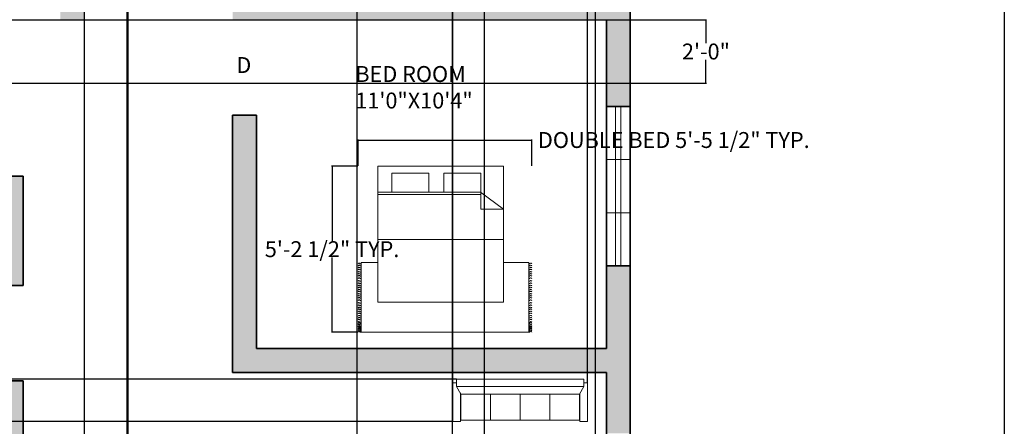
# Model space of a CAD drawing. Units: inches. Extents: x 2552 to 3196, y 4736 to 5443.
# Tile 4 of 8: x 2824 to 3196, y 4983 to 5136. Entities that reach past the tile are written whole.
import ezdxf

# ---------------------------------------------------------------- set-up
doc = ezdxf.new("R2010")
doc.units = ezdxf.units.IN
doc.header["$MEASUREMENT"] = 0
for name, color, linetype, lineweight in [('A-ANNO-DIMS', 2, 'Continuous', 18), ('A-ANNO-TTLB', 7, 'Continuous', 25), ('A-AREA-IDEN', 7, 'Continuous', 18), ('A-DOOR-IDEN', 7, 'Continuous', 18), ('A-FURN', 8, 'Continuous', 18), ('A-GLAZ', 4, 'Continuous', 18), ('A-WALL', 7, 'Continuous', 35)]:
    doc.layers.add(name, color=color, linetype=linetype, lineweight=lineweight)
doc.layers.add('A-WALL-PATT', color=30, linetype='Continuous', lineweight=13, true_color=0xf8991e)
doc.styles.get("Standard").update_dxf_attribs({"font": 'arial.ttf'})
doc.dimstyles.get("Standard").update_dxf_attribs({"dimtxt": 6, "dimasz": 0.18, "dimexe": 0.18, "dimexo": 0.0625, "dimgap": 0.09, "dimtad": 0, "dimtih": 1, "dimtoh": 1, "dimdec": 1, "dimzin": 0, "dimdsep": 46, "dimlunit": 3, "dimtxsty": 'Standard', "dimcen": 0.09, "dimadec": 0, "dimazin": 0, "dimtfac": 1, "dimtdec": 1, "dimtofl": 0, "dimtmove": 0, "dimatfit": 3, "dimfxl": 1, "dimtolj": 1, "dimtzin": 0, "dimarcsym": 0})

# ---------------------------------------------------------------- blocks, each defined once
blk = doc.blocks.new('WIN-60IN-THREE-LIGHT')
for p, q in [((60, 9), (0, 9)), ((20, 9), (20, 0)), ((40, 0), (40, 9)), ((60, 5.5), (0, 5.5)), ((0, 3.5), (60, 3.5)), ((0, 0), (60, 0))]:
    blk.add_line(p, q)
blk = doc.blocks.new('BED-DOUBLE')
for p, q in [((46.16, 52.82), (7.4, 52.82)), ((46.22, 52), (7.4, 52)), ((46.16, 52.82), (54.77, 46.47)), ((46.22, 52.82), (46.22, 46.47)), ((46.22, 46.47), (54.77, 46.47)), ((54.83, 34.96), (7.4, 34.96)), ((1.13, 0), (1.13, 26.37)), ((1.13, 26.37), (7.43, 26.37)), ((54.83, 26.37), (64.37, 26.37)), ((64.37, 26.37), (64.37, 0)), ((64.37, 0), (1.13, 0))]:
    blk.add_line(p, q)
for points in [[(54.83, 62.68), (54.83, 11.36), (7.4, 11.36), (7.4, 62.68)], [(26.65, 59.98), (26.65, 52.82), (12.75, 52.82), (12.75, 59.98)], [(46.22, 59.98), (46.22, 52.82), (32.32, 52.82), (32.32, 59.98)]]:
    blk.add_lwpolyline(points, close=True)
for points, knots in [([(0, 25.83), (0.1, 25.96), (0.29, 26.2), (0.63, 25.96), (0.91, 25.78), (1.06, 25.89), (1.13, 25.94)], [0, 0, 0, 0, 0.400747, 0.791423, 1.067667, 1.29709, 1.29709, 1.29709, 1.29709]), ([(65.48, 25.83), (65.39, 25.96), (65.19, 26.2), (64.85, 25.96), (64.57, 25.78), (64.42, 25.89), (64.36, 25.94)], [0, 0, 0, 0, 0.400747, 0.791423, 1.067667, 1.29709, 1.29709, 1.29709, 1.29709]), ([(0, 25.06), (0.1, 25.18), (0.29, 25.42), (0.63, 25.18), (0.91, 25), (1.06, 25.11), (1.13, 25.16)], [0, 0, 0, 0, 0.400747, 0.791423, 1.067667, 1.29709, 1.29709, 1.29709, 1.29709]), ([(0, 24.24), (0.1, 24.36), (0.29, 24.6), (0.63, 24.36), (0.91, 24.19), (1.06, 24.29), (1.13, 24.34)], [0, 0, 0, 0, 0.400747, 0.791423, 1.067667, 1.29709, 1.29709, 1.29709, 1.29709]), ([(0, 23.51), (0.1, 23.63), (0.29, 23.87), (0.63, 23.63), (0.91, 23.46), (1.06, 23.57), (1.13, 23.62)], [0, 0, 0, 0, 0.400747, 0.791423, 1.067667, 1.29709, 1.29709, 1.29709, 1.29709]), ([(0, 22.63), (0.1, 22.75), (0.29, 22.99), (0.63, 22.75), (0.91, 22.58), (1.06, 22.68), (1.13, 22.73)], [0, 0, 0, 0, 0.400747, 0.791423, 1.067667, 1.29709, 1.29709, 1.29709, 1.29709]), ([(65.48, 25.06), (65.39, 25.18), (65.19, 25.42), (64.85, 25.18), (64.57, 25), (64.42, 25.11), (64.36, 25.16)], [0, 0, 0, 0, 0.400747, 0.791423, 1.067667, 1.29709, 1.29709, 1.29709, 1.29709]), ([(65.48, 24.24), (65.39, 24.36), (65.19, 24.6), (64.85, 24.36), (64.57, 24.19), (64.42, 24.29), (64.36, 24.34)], [0, 0, 0, 0, 0.400747, 0.791423, 1.067667, 1.29709, 1.29709, 1.29709, 1.29709]), ([(65.48, 23.51), (65.39, 23.63), (65.19, 23.87), (64.85, 23.63), (64.57, 23.46), (64.42, 23.57), (64.36, 23.62)], [0, 0, 0, 0, 0.400747, 0.791423, 1.067667, 1.29709, 1.29709, 1.29709, 1.29709]), ([(65.48, 22.63), (65.39, 22.75), (65.19, 22.99), (64.85, 22.75), (64.57, 22.58), (64.42, 22.68), (64.36, 22.73)], [0, 0, 0, 0, 0.400747, 0.791423, 1.067667, 1.29709, 1.29709, 1.29709, 1.29709]), ([(0, 21.88), (0.1, 22), (0.29, 22.24), (0.63, 22), (0.91, 21.83), (1.06, 21.93), (1.13, 21.98)], [0, 0, 0, 0, 0.400747, 0.791423, 1.067667, 1.29709, 1.29709, 1.29709, 1.29709]), ([(0, 21.15), (0.1, 21.27), (0.29, 21.51), (0.63, 21.27), (0.91, 21.1), (1.06, 21.2), (1.13, 21.25)], [0, 0, 0, 0, 0.400747, 0.791423, 1.067667, 1.29709, 1.29709, 1.29709, 1.29709]), ([(0, 20.27), (0.1, 20.39), (0.29, 20.63), (0.63, 20.39), (0.91, 20.22), (1.06, 20.32), (1.13, 20.37)], [0, 0, 0, 0, 0.400747, 0.791423, 1.067667, 1.29709, 1.29709, 1.29709, 1.29709]), ([(0, 19.23), (0.1, 19.35), (0.29, 19.59), (0.63, 19.35), (0.91, 19.18), (1.06, 19.29), (1.13, 19.33)], [0, 0, 0, 0, 0.400747, 0.791423, 1.067667, 1.29709, 1.29709, 1.29709, 1.29709]), ([(0, 18.35), (0.1, 18.47), (0.29, 18.71), (0.63, 18.47), (0.91, 18.3), (1.06, 18.4), (1.13, 18.45)], [0, 0, 0, 0, 0.400747, 0.791423, 1.067667, 1.29709, 1.29709, 1.29709, 1.29709]), ([(65.48, 21.88), (65.39, 22), (65.19, 22.24), (64.85, 22), (64.57, 21.83), (64.42, 21.93), (64.36, 21.98)], [0, 0, 0, 0, 0.400747, 0.791423, 1.067667, 1.29709, 1.29709, 1.29709, 1.29709]), ([(65.48, 21.15), (65.39, 21.27), (65.19, 21.51), (64.85, 21.27), (64.57, 21.1), (64.42, 21.2), (64.36, 21.25)], [0, 0, 0, 0, 0.400747, 0.791423, 1.067667, 1.29709, 1.29709, 1.29709, 1.29709]), ([(65.48, 20.27), (65.39, 20.39), (65.19, 20.63), (64.85, 20.39), (64.57, 20.22), (64.42, 20.32), (64.36, 20.37)], [0, 0, 0, 0, 0.400747, 0.791423, 1.067667, 1.29709, 1.29709, 1.29709, 1.29709]), ([(65.48, 19.23), (65.39, 19.35), (65.19, 19.59), (64.85, 19.35), (64.57, 19.18), (64.42, 19.29), (64.36, 19.33)], [0, 0, 0, 0, 0.400747, 0.791423, 1.067667, 1.29709, 1.29709, 1.29709, 1.29709]), ([(65.48, 18.35), (65.39, 18.47), (65.19, 18.71), (64.85, 18.47), (64.57, 18.3), (64.42, 18.4), (64.36, 18.45)], [0, 0, 0, 0, 0.400747, 0.791423, 1.067667, 1.29709, 1.29709, 1.29709, 1.29709]), ([(0, 17.53), (0.1, 17.65), (0.29, 17.89), (0.63, 17.65), (0.91, 17.48), (1.06, 17.59), (1.13, 17.64)], [0, 0, 0, 0, 0.400747, 0.791423, 1.067667, 1.29709, 1.29709, 1.29709, 1.29709]), ([(0, 16.76), (0.1, 16.88), (0.29, 17.12), (0.63, 16.88), (0.91, 16.7), (1.06, 16.81), (1.13, 16.86)], [0, 0, 0, 0, 0.400747, 0.791423, 1.067667, 1.29709, 1.29709, 1.29709, 1.29709]), ([(0, 15.94), (0.1, 16.06), (0.29, 16.3), (0.63, 16.06), (0.91, 15.89), (1.06, 15.99), (1.13, 16.04)], [0, 0, 0, 0, 0.400747, 0.791423, 1.067667, 1.29709, 1.29709, 1.29709, 1.29709]), ([(0, 15.21), (0.1, 15.33), (0.29, 15.57), (0.63, 15.33), (0.91, 15.16), (1.06, 15.27), (1.13, 15.31)], [0, 0, 0, 0, 0.400747, 0.791423, 1.067667, 1.29709, 1.29709, 1.29709, 1.29709]), ([(65.48, 17.53), (65.39, 17.65), (65.19, 17.89), (64.85, 17.65), (64.57, 17.48), (64.42, 17.59), (64.36, 17.64)], [0, 0, 0, 0, 0.400747, 0.791423, 1.067667, 1.29709, 1.29709, 1.29709, 1.29709]), ([(65.48, 16.76), (65.39, 16.88), (65.19, 17.12), (64.85, 16.88), (64.57, 16.7), (64.42, 16.81), (64.36, 16.86)], [0, 0, 0, 0, 0.400747, 0.791423, 1.067667, 1.29709, 1.29709, 1.29709, 1.29709]), ([(65.48, 15.94), (65.39, 16.06), (65.19, 16.3), (64.85, 16.06), (64.57, 15.89), (64.42, 15.99), (64.36, 16.04)], [0, 0, 0, 0, 0.400747, 0.791423, 1.067667, 1.29709, 1.29709, 1.29709, 1.29709]), ([(65.48, 15.21), (65.39, 15.33), (65.19, 15.57), (64.85, 15.33), (64.57, 15.16), (64.42, 15.27), (64.36, 15.31)], [0, 0, 0, 0, 0.400747, 0.791423, 1.067667, 1.29709, 1.29709, 1.29709, 1.29709]), ([(0, 14.33), (0.1, 14.45), (0.29, 14.69), (0.63, 14.45), (0.91, 14.28), (1.06, 14.38), (1.13, 14.43)], [0, 0, 0, 0, 0.400747, 0.791423, 1.067667, 1.29709, 1.29709, 1.29709, 1.29709]), ([(0, 13.58), (0.1, 13.7), (0.29, 13.94), (0.63, 13.7), (0.91, 13.53), (1.06, 13.63), (1.13, 13.68)], [0, 0, 0, 0, 0.400747, 0.791423, 1.067667, 1.29709, 1.29709, 1.29709, 1.29709]), ([(0, 12.85), (0.1, 12.97), (0.29, 13.21), (0.63, 12.97), (0.91, 12.8), (1.06, 12.9), (1.13, 12.95)], [0, 0, 0, 0, 0.400747, 0.791423, 1.067667, 1.29709, 1.29709, 1.29709, 1.29709]), ([(0, 11.97), (0.1, 12.09), (0.29, 12.33), (0.63, 12.09), (0.91, 11.92), (1.06, 12.02), (1.13, 12.07)], [0, 0, 0, 0, 0.400747, 0.791423, 1.067667, 1.29709, 1.29709, 1.29709, 1.29709]), ([(0, 10.93), (0.1, 11.05), (0.29, 11.29), (0.63, 11.05), (0.91, 10.88), (1.06, 10.99), (1.13, 11.03)], [0, 0, 0, 0, 0.400747, 0.791423, 1.067667, 1.29709, 1.29709, 1.29709, 1.29709]), ([(65.48, 14.33), (65.39, 14.45), (65.19, 14.69), (64.85, 14.45), (64.57, 14.28), (64.42, 14.38), (64.36, 14.43)], [0, 0, 0, 0, 0.400747, 0.791423, 1.067667, 1.29709, 1.29709, 1.29709, 1.29709]), ([(65.48, 13.58), (65.39, 13.7), (65.19, 13.94), (64.85, 13.7), (64.57, 13.53), (64.42, 13.63), (64.36, 13.68)], [0, 0, 0, 0, 0.400747, 0.791423, 1.067667, 1.29709, 1.29709, 1.29709, 1.29709]), ([(65.48, 12.85), (65.39, 12.97), (65.19, 13.21), (64.85, 12.97), (64.57, 12.8), (64.42, 12.9), (64.36, 12.95)], [0, 0, 0, 0, 0.400747, 0.791423, 1.067667, 1.29709, 1.29709, 1.29709, 1.29709]), ([(65.48, 11.97), (65.39, 12.09), (65.19, 12.33), (64.85, 12.09), (64.57, 11.92), (64.42, 12.02), (64.36, 12.07)], [0, 0, 0, 0, 0.400747, 0.791423, 1.067667, 1.29709, 1.29709, 1.29709, 1.29709]), ([(65.48, 10.93), (65.39, 11.05), (65.19, 11.29), (64.85, 11.05), (64.57, 10.88), (64.42, 10.99), (64.36, 11.03)], [0, 0, 0, 0, 0.400747, 0.791423, 1.067667, 1.29709, 1.29709, 1.29709, 1.29709]), ([(0, 10.05), (0.1, 10.17), (0.29, 10.41), (0.63, 10.17), (0.91, 10), (1.06, 10.1), (1.13, 10.15)], [0, 0, 0, 0, 0.400747, 0.791423, 1.067667, 1.29709, 1.29709, 1.29709, 1.29709]), ([(0, 9.23), (0.1, 9.35), (0.29, 9.59), (0.63, 9.35), (0.91, 9.18), (1.06, 9.29), (1.13, 9.33)], [0, 0, 0, 0, 0.400747, 0.791423, 1.067667, 1.29709, 1.29709, 1.29709, 1.29709]), ([(0, 8.54), (0.1, 8.66), (0.29, 8.9), (0.63, 8.66), (0.91, 8.49), (1.06, 8.6), (1.13, 8.65)], [0, 0, 0, 0, 0.400747, 0.791423, 1.067667, 1.29709, 1.29709, 1.29709, 1.29709]), ([(0, 7.73), (0.1, 7.85), (0.29, 8.09), (0.63, 7.85), (0.91, 7.67), (1.06, 7.78), (1.13, 7.83)], [0, 0, 0, 0, 0.400747, 0.791423, 1.067667, 1.29709, 1.29709, 1.29709, 1.29709]), ([(65.48, 10.05), (65.39, 10.17), (65.19, 10.41), (64.85, 10.17), (64.57, 10), (64.42, 10.1), (64.36, 10.15)], [0, 0, 0, 0, 0.400747, 0.791423, 1.067667, 1.29709, 1.29709, 1.29709, 1.29709]), ([(65.48, 9.23), (65.39, 9.35), (65.19, 9.59), (64.85, 9.35), (64.57, 9.18), (64.42, 9.29), (64.36, 9.33)], [0, 0, 0, 0, 0.400747, 0.791423, 1.067667, 1.29709, 1.29709, 1.29709, 1.29709]), ([(65.48, 8.54), (65.39, 8.66), (65.19, 8.9), (64.85, 8.66), (64.57, 8.49), (64.42, 8.6), (64.36, 8.65)], [0, 0, 0, 0, 0.400747, 0.791423, 1.067667, 1.29709, 1.29709, 1.29709, 1.29709]), ([(65.48, 7.73), (65.39, 7.85), (65.19, 8.09), (64.85, 7.85), (64.57, 7.67), (64.42, 7.78), (64.36, 7.83)], [0, 0, 0, 0, 0.400747, 0.791423, 1.067667, 1.29709, 1.29709, 1.29709, 1.29709]), ([(0, 7), (0.1, 7.12), (0.29, 7.36), (0.63, 7.12), (0.91, 6.95), (1.06, 7.05), (1.13, 7.1)], [0, 0, 0, 0, 0.400747, 0.791423, 1.067667, 1.29709, 1.29709, 1.29709, 1.29709]), ([(0, 6.12), (0.1, 6.24), (0.29, 6.48), (0.63, 6.24), (0.91, 6.06), (1.06, 6.17), (1.13, 6.22)], [0, 0, 0, 0, 0.400747, 0.791423, 1.067667, 1.29709, 1.29709, 1.29709, 1.29709]), ([(0, 5.36), (0.1, 5.49), (0.29, 5.72), (0.63, 5.49), (0.91, 5.31), (1.06, 5.42), (1.13, 5.47)], [0, 0, 0, 0, 0.400747, 0.791423, 1.067667, 1.29709, 1.29709, 1.29709, 1.29709]), ([(0, 4.64), (0.1, 4.76), (0.29, 5), (0.63, 4.76), (0.91, 4.58), (1.06, 4.69), (1.13, 4.74)], [0, 0, 0, 0, 0.400747, 0.791423, 1.067667, 1.29709, 1.29709, 1.29709, 1.29709]), ([(0, 3.75), (0.1, 3.87), (0.29, 4.11), (0.63, 3.87), (0.91, 3.7), (1.06, 3.81), (1.13, 3.86)], [0, 0, 0, 0, 0.400747, 0.791423, 1.067667, 1.29709, 1.29709, 1.29709, 1.29709]), ([(65.48, 7), (65.39, 7.12), (65.19, 7.36), (64.85, 7.12), (64.57, 6.95), (64.42, 7.05), (64.36, 7.1)], [0, 0, 0, 0, 0.400747, 0.791423, 1.067667, 1.29709, 1.29709, 1.29709, 1.29709]), ([(65.48, 6.12), (65.39, 6.24), (65.19, 6.48), (64.85, 6.24), (64.57, 6.06), (64.42, 6.17), (64.36, 6.22)], [0, 0, 0, 0, 0.400747, 0.791423, 1.067667, 1.29709, 1.29709, 1.29709, 1.29709]), ([(65.48, 5.36), (65.39, 5.49), (65.19, 5.72), (64.85, 5.49), (64.57, 5.31), (64.42, 5.42), (64.36, 5.47)], [0, 0, 0, 0, 0.400747, 0.791423, 1.067667, 1.29709, 1.29709, 1.29709, 1.29709]), ([(65.48, 4.64), (65.39, 4.76), (65.19, 5), (64.85, 4.76), (64.58, 4.59), (64.43, 4.69), (64.37, 4.73)], [0, 0, 0, 0, 0.400747, 0.791423, 1.067667, 1.283686, 1.283686, 1.283686, 1.283686]), ([(65.48, 3.75), (65.39, 3.87), (65.19, 4.11), (64.85, 3.88), (64.58, 3.7), (64.43, 3.8), (64.37, 3.85)], [0, 0, 0, 0, 0.400747, 0.791423, 1.067667, 1.283686, 1.283686, 1.283686, 1.283686]), ([(0, 3.32), (0.1, 3.45), (0.29, 3.7), (0.63, 3.44), (0.91, 3.27), (1.06, 3.38), (1.13, 3.43)], [0, 0, 0, 0, 0.407265, 0.802015, 1.07826, 1.307683, 1.307683, 1.307683, 1.307683]), ([(0, 2.76), (0.1, 2.88), (0.29, 3.12), (0.63, 2.88), (0.91, 2.71), (1.06, 2.81), (1.13, 2.86)], [0, 0, 0, 0, 0.400747, 0.791423, 1.067667, 1.29709, 1.29709, 1.29709, 1.29709]), ([(0, 2.18), (0.1, 2.31), (0.29, 2.54), (0.63, 2.31), (0.91, 2.13), (1.06, 2.24), (1.13, 2.29)], [0, 0, 0, 0, 0.400747, 0.791423, 1.067667, 1.29709, 1.29709, 1.29709, 1.29709]), ([(0, 1.88), (0.1, 2), (0.29, 2.24), (0.63, 2), (0.91, 1.82), (1.06, 1.93), (1.13, 1.98)], [0, 0, 0, 0, 0.400747, 0.791423, 1.067667, 1.29709, 1.29709, 1.29709, 1.29709]), ([(0, 1.46), (0.1, 1.58), (0.29, 1.82), (0.63, 1.58), (0.91, 1.4), (1.06, 1.51), (1.13, 1.56)], [0, 0, 0, 0, 0.400747, 0.791423, 1.067667, 1.29709, 1.29709, 1.29709, 1.29709]), ([(0, 1.06), (0.1, 1.18), (0.29, 1.42), (0.63, 1.18), (0.91, 1.01), (1.06, 1.11), (1.13, 1.16)], [0, 0, 0, 0, 0.400747, 0.791423, 1.067667, 1.29709, 1.29709, 1.29709, 1.29709]), ([(0, 0.57), (0.1, 0.7), (0.29, 0.93), (0.63, 0.7), (0.91, 0.52), (1.06, 0.63), (1.13, 0.68)], [0, 0, 0, 0, 0.400747, 0.791423, 1.067667, 1.29709, 1.29709, 1.29709, 1.29709]), ([(0, 0.07), (0.1, 0.19), (0.29, 0.43), (0.63, 0.19), (0.91, 0.02), (1.06, 0.13), (1.13, 0.17)], [0, 0, 0, 0, 0.400747, 0.791423, 1.067667, 1.29709, 1.29709, 1.29709, 1.29709]), ([(65.48, 1.43), (65.39, 1.55), (65.19, 1.79), (64.85, 1.55), (64.57, 1.38), (64.42, 1.48), (64.36, 1.53)], [0, 0, 0, 0, 0.400747, 0.791423, 1.067667, 1.29709, 1.29709, 1.29709, 1.29709]), ([(65.48, 1.03), (65.39, 1.15), (65.19, 1.39), (64.85, 1.15), (64.57, 0.98), (64.42, 1.09), (64.36, 1.13)], [0, 0, 0, 0, 0.400747, 0.791423, 1.067667, 1.29709, 1.29709, 1.29709, 1.29709]), ([(65.48, 0.55), (65.39, 0.67), (65.19, 0.91), (64.85, 0.67), (64.57, 0.49), (64.42, 0.6), (64.36, 0.65)], [0, 0, 0, 0, 0.400747, 0.791423, 1.067667, 1.29709, 1.29709, 1.29709, 1.29709]), ([(65.48, 0.07), (65.39, 0.19), (65.19, 0.43), (64.85, 0.19), (64.57, 0.02), (64.42, 0.13), (64.36, 0.17)], [0, 0, 0, 0, 0.400747, 0.791423, 1.067667, 1.29709, 1.29709, 1.29709, 1.29709]), ([(65.48, 3.32), (65.39, 3.45), (65.19, 3.69), (64.85, 3.45), (64.58, 3.27), (64.43, 3.37), (64.37, 3.42)], [0, 0, 0, 0, 0.402903, 0.794912, 1.071156, 1.287177, 1.287177, 1.287177, 1.287177]), ([(65.48, 2.73), (65.39, 2.85), (65.19, 3.09), (64.85, 2.85), (64.58, 2.68), (64.43, 2.78), (64.37, 2.82)], [0, 0, 0, 0, 0.400747, 0.791423, 1.067667, 1.283686, 1.283686, 1.283686, 1.283686]), ([(65.48, 2.16), (65.39, 2.28), (65.19, 2.52), (64.85, 2.28), (64.58, 2.11), (64.43, 2.21), (64.37, 2.25)], [0, 0, 0, 0, 0.400747, 0.791423, 1.067667, 1.283686, 1.283686, 1.283686, 1.283686]), ([(65.48, 1.85), (65.39, 1.97), (65.19, 2.21), (64.85, 1.97), (64.58, 1.8), (64.43, 1.9), (64.37, 1.94)], [0, 0, 0, 0, 0.400747, 0.791423, 1.067667, 1.283686, 1.283686, 1.283686, 1.283686])]:
    blk.add_open_spline(points, degree=3, knots=knots)
blk = doc.blocks.new('*D13')
at = {"layer": 'A-ANNO-DIMS', "color": 0, "lineweight": -2, "transparency": 16777216}
for p, q in [((2952.04, 5081.18), (2952.04, 5091.12)), ((2952.22, 5090.94), (3017.34, 5090.94)), ((3017.52, 5081.18), (3017.52, 5091.12)), ((3017.52, 5090.94), (3017.7, 5090.94))]:
    blk.add_line(p, q, dxfattribs=at)
at = {"layer": 'A-ANNO-DIMS', "color": 0, "transparency": 16777216}
for points in [[(2952.22, 5090.97), (2952.22, 5090.91), (2952.04, 5090.94)], [(3017.34, 5090.97), (3017.34, 5090.91), (3017.52, 5090.94)]]:
    blk.add_solid(points, dxfattribs=at)
at = {"layer": 'Defpoints', "color": 0, "transparency": 16777216}
for p in [(3017.52, 5090.94), (2952.04, 5081.12), (3017.52, 5081.12)]:
    blk.add_point(p, dxfattribs=at)
at = {"layer": 'A-ANNO-DIMS', "color": 0, "transparency": 16777216, "insert": (3071.1, 5090.94), "char_height": 6, "attachment_point": 5}
blk.add_mtext('\\A1;DOUBLE BED 5\'-5 1/2" TYP.', dxfattribs=at)
blk = doc.blocks.new('*D14')
at = {"layer": 'A-ANNO-DIMS', "color": 0, "lineweight": -2, "transparency": 16777216}
for p, q in [((2951.97, 5081.12), (2942.03, 5081.12)), ((2942.21, 5080.94), (2942.21, 5052.97)), ((2942.21, 5018.62), (2942.21, 5046.59)), ((2951.97, 5018.44), (2942.03, 5018.44))]:
    blk.add_line(p, q, dxfattribs=at)
at = {"layer": 'A-ANNO-DIMS', "color": 0, "transparency": 16777216}
for points in [[(2942.18, 5080.94), (2942.24, 5080.94), (2942.21, 5081.12)], [(2942.18, 5018.62), (2942.24, 5018.62), (2942.21, 5018.44)]]:
    blk.add_solid(points, dxfattribs=at)
at = {"layer": 'Defpoints', "color": 0, "transparency": 16777216}
for p in [(2942.21, 5081.12), (2952.04, 5081.12), (2952.04, 5018.44)]:
    blk.add_point(p, dxfattribs=at)
at = {"layer": 'A-ANNO-DIMS', "color": 0, "transparency": 16777216, "insert": (2942.21, 5049.78), "char_height": 6, "attachment_point": 5}
blk.add_mtext('\\A1;5\'-2 1/2" TYP.', dxfattribs=at)
blk = doc.blocks.new('*D24')
at = {"layer": 'A-ANNO-DIMS', "color": 0, "lineweight": -2, "transparency": 16777216}
for p, q in [((2951.66, 4886.38), (2951.66, 5320.05)), ((2951.84, 5319.87), (2961.59, 5319.87)), ((2987.48, 5319.87), (2977.72, 5319.87)), ((2987.66, 4886.38), (2987.66, 5320.05))]:
    blk.add_line(p, q, dxfattribs=at)
at = {"layer": 'A-ANNO-DIMS', "color": 0, "transparency": 16777216}
for points in [[(2951.84, 5319.9), (2951.84, 5319.84), (2951.66, 5319.87)], [(2987.48, 5319.9), (2987.48, 5319.84), (2987.66, 5319.87)]]:
    blk.add_solid(points, dxfattribs=at)
at = {"layer": 'Defpoints', "color": 0, "transparency": 16777216}
for p in [(2987.66, 5319.87), (2951.66, 4886.32), (2987.66, 4886.32)]:
    blk.add_point(p, dxfattribs=at)
at = {"layer": 'A-ANNO-DIMS', "color": 0, "transparency": 16777216, "insert": (2969.66, 5319.87), "char_height": 6, "attachment_point": 5}
blk.add_mtext('\\A1;3\'-0"', dxfattribs=at)
blk = doc.blocks.new('*D26')
at = {"layer": 'A-ANNO-DIMS', "color": 0, "lineweight": -2, "transparency": 16777216}
for p, q in [((2803.72, 5136.32), (3083.39, 5136.32)), ((3083.21, 5136.14), (3083.21, 5127.47)), ((3083.21, 5112.5), (3083.21, 5121.16)), ((2773.72, 5112.32), (3083.39, 5112.32))]:
    blk.add_line(p, q, dxfattribs=at)
at = {"layer": 'A-ANNO-DIMS', "color": 0, "transparency": 16777216}
for points in [[(3083.18, 5136.14), (3083.24, 5136.14), (3083.21, 5136.32)], [(3083.18, 5112.5), (3083.24, 5112.5), (3083.21, 5112.32)]]:
    blk.add_solid(points, dxfattribs=at)
at = {"layer": 'Defpoints', "color": 0, "transparency": 16777216}
for p in [(2803.66, 5136.32), (2773.66, 5112.32), (3083.21, 5112.32)]:
    blk.add_point(p, dxfattribs=at)
at = {"layer": 'A-ANNO-DIMS', "color": 0, "transparency": 16777216, "insert": (3083.21, 5124.32), "char_height": 6, "attachment_point": 5}
blk.add_mtext('\\A1;2\'-0"', dxfattribs=at)
blk = doc.blocks.new('*D27')
at = {"layer": 'A-ANNO-DIMS', "color": 0, "lineweight": -2, "transparency": 16777216}
for p, q in [((2999.73, 4817.38), (2999.73, 5320.05)), ((2999.91, 5319.87), (3012.6, 5319.87)), ((3041.41, 5319.87), (3028.73, 5319.87)), ((3041.59, 4817.38), (3041.59, 5320.05))]:
    blk.add_line(p, q, dxfattribs=at)
at = {"layer": 'A-ANNO-DIMS', "color": 0, "transparency": 16777216}
for points in [[(2999.91, 5319.9), (2999.91, 5319.84), (2999.73, 5319.87)], [(3041.41, 5319.9), (3041.41, 5319.84), (3041.59, 5319.87)]]:
    blk.add_solid(points, dxfattribs=at)
at = {"layer": 'Defpoints', "color": 0, "transparency": 16777216}
for p in [(3041.59, 5319.87), (2999.73, 4817.32), (3041.59, 4817.32)]:
    blk.add_point(p, dxfattribs=at)
at = {"layer": 'A-ANNO-DIMS', "color": 0, "transparency": 16777216, "insert": (3020.66, 5319.87), "char_height": 6, "attachment_point": 5}
blk.add_mtext('\\A1;3\'-6"', dxfattribs=at)
blk = doc.blocks.new('*D31')
at = {"layer": 'A-ANNO-DIMS', "color": 0, "lineweight": -2, "transparency": 16777216}
for p, q in [((2848.66, 5282.26), (2848.66, 4759.59)), ((2865.22, 5282.26), (2865.22, 4759.59)), ((2848.84, 4759.77), (2865.04, 4759.77)), ((2865.22, 4759.77), (2865.4, 4759.77))]:
    blk.add_line(p, q, dxfattribs=at)
at = {"layer": 'A-ANNO-DIMS', "color": 0, "transparency": 16777216}
for points in [[(2848.84, 4759.8), (2848.84, 4759.74), (2848.66, 4759.77)], [(2865.04, 4759.8), (2865.04, 4759.74), (2865.22, 4759.77)]]:
    blk.add_solid(points, dxfattribs=at)
at = {"layer": 'Defpoints', "color": 0, "transparency": 16777216}
for p in [(2848.66, 5282.32), (2865.22, 5282.32), (2865.22, 4759.77)]:
    blk.add_point(p, dxfattribs=at)
at = {"layer": 'A-ANNO-DIMS', "color": 0, "transparency": 16777216, "insert": (2880.18, 4759.77), "char_height": 6, "attachment_point": 5}
blk.add_mtext('\\A1;1\'-4 1/2"', dxfattribs=at)
blk = doc.blocks.new('*D32')
at = {"layer": 'A-ANNO-DIMS', "color": 0, "lineweight": -2, "transparency": 16777216}
for p, q in [((2864.75, 5194.1), (2864.75, 4759.59)), ((2848.66, 5191.26), (2848.66, 4759.59)), ((2848.48, 4759.77), (2848.3, 4759.77)), ((2864.93, 4759.77), (2865.11, 4759.77))]:
    blk.add_line(p, q, dxfattribs=at)
at = {"layer": 'A-ANNO-DIMS', "color": 0, "transparency": 16777216}
for points in [[(2848.48, 4759.8), (2848.48, 4759.74), (2848.66, 4759.77)], [(2864.93, 4759.8), (2864.93, 4759.74), (2864.75, 4759.77)]]:
    blk.add_solid(points, dxfattribs=at)
at = {"layer": 'Defpoints', "color": 0, "transparency": 16777216}
for p in [(2864.75, 5194.17), (2848.66, 5191.32), (2864.75, 4759.77)]:
    blk.add_point(p, dxfattribs=at)
at = {"layer": 'A-ANNO-DIMS', "color": 0, "transparency": 16777216, "insert": (2856.7, 4759.77), "char_height": 6, "attachment_point": 5}
blk.add_mtext('\\A1;1\'-4"', dxfattribs=at)
blk = doc.blocks.new('*D33')
at = {"layer": 'A-ANNO-DIMS', "color": 0, "lineweight": -2, "transparency": 16777216}
for p, q in [((2987.78, 4999.44), (2987.78, 5320.05)), ((2987.96, 5319.87), (2997.97, 5319.87)), ((3038.33, 5319.87), (3028.32, 5319.87)), ((3038.51, 4999.44), (3038.51, 5320.05))]:
    blk.add_line(p, q, dxfattribs=at)
at = {"layer": 'A-ANNO-DIMS', "color": 0, "transparency": 16777216}
for points in [[(2987.96, 5319.9), (2987.96, 5319.84), (2987.78, 5319.87)], [(3038.33, 5319.9), (3038.33, 5319.84), (3038.51, 5319.87)]]:
    blk.add_solid(points, dxfattribs=at)
at = {"layer": 'Defpoints', "color": 0, "transparency": 16777216}
for p in [(3038.51, 5319.87), (2987.78, 4999.37), (3038.51, 4999.37)]:
    blk.add_point(p, dxfattribs=at)
at = {"layer": 'A-ANNO-DIMS', "color": 0, "transparency": 16777216, "insert": (3013.14, 5319.87), "char_height": 6, "attachment_point": 5}
blk.add_mtext('\\A1;4\'-2 1/2"', dxfattribs=at)
blk = doc.blocks.new('*D34')
at = {"layer": 'A-ANNO-DIMS', "color": 0, "lineweight": -2, "transparency": 16777216}
for p, q in [((2989.13, 5000.78), (2662.93, 5000.78)), ((2663.11, 5000.6), (2663.11, 4995.9)), ((2663.11, 4984.99), (2663.11, 4989.7)), ((2987.72, 4984.81), (2662.93, 4984.81))]:
    blk.add_line(p, q, dxfattribs=at)
at = {"layer": 'A-ANNO-DIMS', "color": 0, "transparency": 16777216}
for points in [[(2663.08, 5000.6), (2663.14, 5000.6), (2663.11, 5000.78)], [(2663.08, 4984.99), (2663.14, 4984.99), (2663.11, 4984.81)]]:
    blk.add_solid(points, dxfattribs=at)
at = {"layer": 'Defpoints', "color": 0, "transparency": 16777216}
for p in [(2663.11, 5000.78), (2989.19, 5000.78), (2987.78, 4984.81)]:
    blk.add_point(p, dxfattribs=at)
at = {"layer": 'A-ANNO-DIMS', "color": 0, "transparency": 16777216, "insert": (2663.11, 4992.8), "char_height": 6, "attachment_point": 5}
blk.add_mtext('\\A1;1\'-4"', dxfattribs=at)

msp = doc.modelspace()

# ---------------------------------------------------------------- hatches: boundary and pattern name
at = {"layer": 'A-WALL-PATT'}
h = msp.add_hatch(color=256, dxfattribs=at)
h.dxf.hatch_style = 1
h.paths.add_polyline_path([(2700.66, 5282.32), (2732.91, 5282.32), (2732.91, 5291.32), (2691.66, 5291.32), (2691.66, 5248.4), (2700.66, 5248.4)])
h.paths.add_polyline_path([(2865.22, 5291.32), (2792.91, 5291.32), (2792.91, 5282.32), (2839.66, 5282.32), (2839.66, 5136.32), (2848.66, 5136.32), (2848.66, 5182.32), (2913.66, 5182.32), (2913.66, 5246.32), (2904.66, 5246.32), (2904.66, 5191.32), (2848.66, 5191.32), (2848.66, 5282.32), (2865.22, 5282.32)])
h.paths.add_polyline_path([(2946.08, 5291.32), (2889.22, 5291.32), (2889.22, 5282.32), (2946.08, 5282.32)])
h.paths.add_polyline_path([(3054.66, 5291.32), (3006.08, 5291.32), (3006.08, 5282.32), (3045.66, 5282.32), (3045.66, 5249.18), (3054.66, 5249.18)])
h.paths.add_polyline_path([(3054.66, 5189.18), (3045.66, 5189.18), (3045.66, 5145.32), (2904.66, 5145.32), (2904.66, 5136.32), (3045.66, 5136.32), (3045.66, 5103.54), (3054.66, 5103.54)])
h.paths.add_polyline_path([(3054.66, 5043.54), (3045.66, 5043.54), (3045.66, 5012.32), (2913.66, 5012.32), (2913.66, 5100.32), (2904.66, 5100.32), (2904.66, 5003.32), (3045.66, 5003.32), (3045.66, 4980.34), (3054.66, 4980.34)])
h.paths.add_polyline_path([(3054.66, 4920.34), (3045.66, 4920.34), (3045.66, 4886.32), (3029.6, 4886.32), (3029.6, 4877.32), (3045.66, 4877.32), (3045.66, 4817.32), (3041.59, 4817.32), (3041.59, 4808.32), (3054.66, 4808.32)])
h.paths.add_polyline_path([(2996.66, 4877.32), (3013.11, 4877.32), (3013.11, 4886.32), (2987.66, 4886.32), (2987.66, 4808.32), (2999.73, 4808.32), (2999.73, 4817.32), (2996.66, 4817.32)])
h.paths.add_polyline_path([(2825.66, 4877.32), (2853.9, 4877.32), (2853.9, 4886.32), (2825.66, 4886.32), (2825.66, 5000.12), (2816.66, 5000.12), (2816.66, 4817.32), (2785.76, 4817.32), (2785.76, 4808.32), (2825.66, 4808.32)])
h.paths.add_polyline_path([(2951.66, 4886.32), (2913.9, 4886.32), (2913.9, 4877.32), (2951.66, 4877.32)])
h.paths.add_polyline_path([(2725.76, 4817.32), (2700.66, 4817.32), (2700.66, 4833.17), (2691.66, 4833.17), (2691.66, 4808.32), (2725.76, 4808.32)])
h.paths.add_polyline_path([(2700.66, 4902.32), (2691.66, 4902.32), (2691.66, 4869.17), (2700.66, 4869.17)])
h.paths.add_polyline_path([(2765.91, 4947.32), (2700.66, 4947.32), (2700.66, 4977.71), (2691.66, 4977.71), (2691.66, 4938.32), (2765.91, 4938.32)])
h.paths.add_polyline_path([(2825.66, 5077.32), (2773.66, 5077.32), (2773.66, 5112.32), (2764.66, 5112.32), (2764.66, 5077.32), (2700.66, 5077.32), (2700.66, 5102.51), (2691.66, 5102.51), (2691.66, 5037.71), (2700.66, 5037.71), (2700.66, 5068.32), (2816.66, 5068.32), (2816.66, 5036.12), (2825.66, 5036.12)])
h.paths.add_polyline_path([(2803.66, 5145.32), (2700.66, 5145.32), (2700.66, 5188.4), (2691.66, 5188.4), (2691.66, 5126.51), (2700.66, 5126.51), (2700.66, 5136.32), (2803.66, 5136.32)])

# ---------------------------------------------------------------- linework, layer by layer
at = {"layer": 'A-ANNO-TTLB'}
msp.add_lwpolyline([(2551.65, 5442.6), (3195.75, 5442.6), (3195.75, 4736.32), (2551.65, 4736.32)], close=True, dxfattribs=at)
at = {"layer": 'A-FURN'}
for p, q in [((2987.78, 4999.37), (2987.78, 4984.81)), ((2989.19, 4999.37), (2987.78, 4999.37)), ((3037.1, 5000.78), (2989.19, 5000.78)), ((2989.19, 4997.97), (2989.19, 5000.78)), ((3037.1, 4997.97), (3037.1, 5000.78)), ((3038.51, 4999.37), (3037.1, 4999.37)), ((3038.51, 4999.37), (3038.51, 4984.81)), ((3037.1, 4997.97), (2989.19, 4997.97)), ((2990.78, 4995.15), (2989.19, 4997.97)), ((2990.6, 4995.55), (2990.6, 4984.81)), ((3001.96, 4985.28), (3001.96, 4995.15)), ((3013.14, 4985.28), (3013.14, 4995.15)), ((3024.33, 4985.28), (3024.33, 4995.15)), ((3037.1, 4997.97), (3035.51, 4995.15)), ((3035.69, 4995.36), (3035.69, 4984.81)), ((2990.6, 4984.81), (2987.78, 4984.81)), ((3035.69, 4984.81), (3038.51, 4984.81))]:
    msp.add_line(p, q, dxfattribs=at)
msp.add_lwpolyline([(3035.51, 4995.15), (2990.78, 4995.15), (2990.78, 4985.28), (3035.51, 4985.28)], close=True, dxfattribs=at)
at = {"layer": 'A-WALL'}
for p, q in [((3054.66, 5291.32), (3054.66, 4808.32)), ((3045.66, 5136.32), (3045.66, 5012.32)), ((3045.66, 5103.54), (3054.66, 5103.54)), ((2904.66, 5100.32), (2913.66, 5100.32)), ((2904.66, 5100.32), (2904.66, 5003.32)), ((2913.66, 5100.32), (2913.66, 5012.32)), ((2773.66, 5077.32), (2825.66, 5077.32)), ((2825.66, 5077.32), (2825.66, 5036.12)), ((3054.66, 5043.54), (3045.66, 5043.54)), ((2816.66, 5036.12), (2825.66, 5036.12)), ((2913.66, 5012.32), (3045.66, 5012.32)), ((2904.66, 5003.32), (3045.66, 5003.32)), ((3045.66, 5003.32), (3045.66, 4886.32)), ((2825.66, 5000.12), (2816.66, 5000.12)), ((2825.66, 5000.12), (2825.66, 4886.32))]:
    msp.add_line(p, q, dxfattribs=at)

# ---------------------------------------------------------------- block references
at = {"layer": 'A-FURN'}
msp.add_blockref('BED-DOUBLE', (2952.04, 5018.44), dxfattribs=at)
at = {"layer": 'A-GLAZ', "rotation": 89.99999999999793}
msp.add_blockref('WIN-60IN-THREE-LIGHT', (3054.66, 5043.54), dxfattribs=at)

# ---------------------------------------------------------------- texts
at = {"layer": 'A-AREA-IDEN', "insert": (2950.97, 5118.83), "char_height": 6, "attachment_point": 1}
msp.add_mtext_dynamic_manual_height_columns('BED ROOM\\P11\'0"X10\'4"', width=67.9916, gutter_width=1, heights=[0], dxfattribs=at)
at = {"layer": 'A-DOOR-IDEN', "insert": (2906.1, 5122.21), "char_height": 6, "attachment_point": 1}
msp.add_mtext_dynamic_manual_height_columns('D', width=10.2167, gutter_width=1, heights=[0], dxfattribs=at)

# ---------------------------------------------------------------- dimensions: what is measured, and where the dimension line sits
at = {"layer": 'A-ANNO-DIMS'}
for base, p1, p2, picture, middle in [((3038.51, 5319.87), (2987.78, 4999.37), (3038.51, 4999.37), '*D33', (3013.14, 5319.87)), ((2987.66, 5319.87), (2951.66, 4886.32), (2987.66, 4886.32), '*D24', (2969.66, 5319.87)), ((3041.59, 5319.87), (2999.73, 4817.32), (3041.59, 4817.32), '*D27', (3020.66, 5319.87)), ((2865.22, 4759.77), (2848.66, 5282.32), (2865.22, 5282.32), '*D31', (2880.18, 4759.77)), ((2864.75, 4759.77), (2848.66, 5191.32), (2864.75, 5194.17), '*D32', (2856.7, 4759.77))]:
    dim = msp.add_linear_dim(base=base, p1=p1, p2=p2, dimstyle='Standard', override={"dimdec": 1, "dimlfac": 1, "dimrnd": 0, "dimzin": 1, "dimdsep": 46, "dimlunit": 4, "dimfrac": 2}, dxfattribs=at)
    dim.commit()
    dim.dimension.update_dxf_attribs({"geometry": picture, "text_midpoint": middle})
for base, p1, p2, picture, middle in [((3083.21, 5112.32), (2803.66, 5136.32), (2773.66, 5112.32), '*D26', (3083.21, 5124.32)), ((2663.11, 5000.78), (2987.78, 4984.81), (2989.19, 5000.78), '*D34', (2663.11, 4992.8))]:
    dim = msp.add_linear_dim(base=base, p1=p1, p2=p2, angle=90, dimstyle='Standard', override={"dimdec": 1, "dimlfac": 1, "dimrnd": 0, "dimzin": 1, "dimdsep": 46, "dimlunit": 4, "dimfrac": 2}, dxfattribs=at)
    dim.commit()
    dim.dimension.update_dxf_attribs({"geometry": picture, "text_midpoint": middle})
dim = msp.add_linear_dim(base=(3017.52, 5090.94), p1=(2952.04, 5081.12), p2=(3017.52, 5081.12), text='DOUBLE BED <> TYP.', dimstyle='Standard', override={"dimdec": 1, "dimlfac": 1, "dimrnd": 0, "dimzin": 1, "dimdsep": 46, "dimlunit": 4, "dimfrac": 2}, dxfattribs=at)
dim.commit()
dim.dimension.update_dxf_attribs({"geometry": '*D13', "text_midpoint": (3071.1, 5090.94)})
dim = msp.add_linear_dim(base=(2942.21, 5081.12), p1=(2952.04, 5018.44), p2=(2952.04, 5081.12), angle=90, text='<> TYP.', dimstyle='Standard', override={"dimdec": 1, "dimlfac": 1, "dimrnd": 0, "dimzin": 1, "dimdsep": 46, "dimlunit": 4, "dimfrac": 2}, dxfattribs=at)
dim.commit()
dim.dimension.update_dxf_attribs({"geometry": '*D14', "text_midpoint": (2942.21, 5049.78)})

doc.saveas('drawing.dxf')
